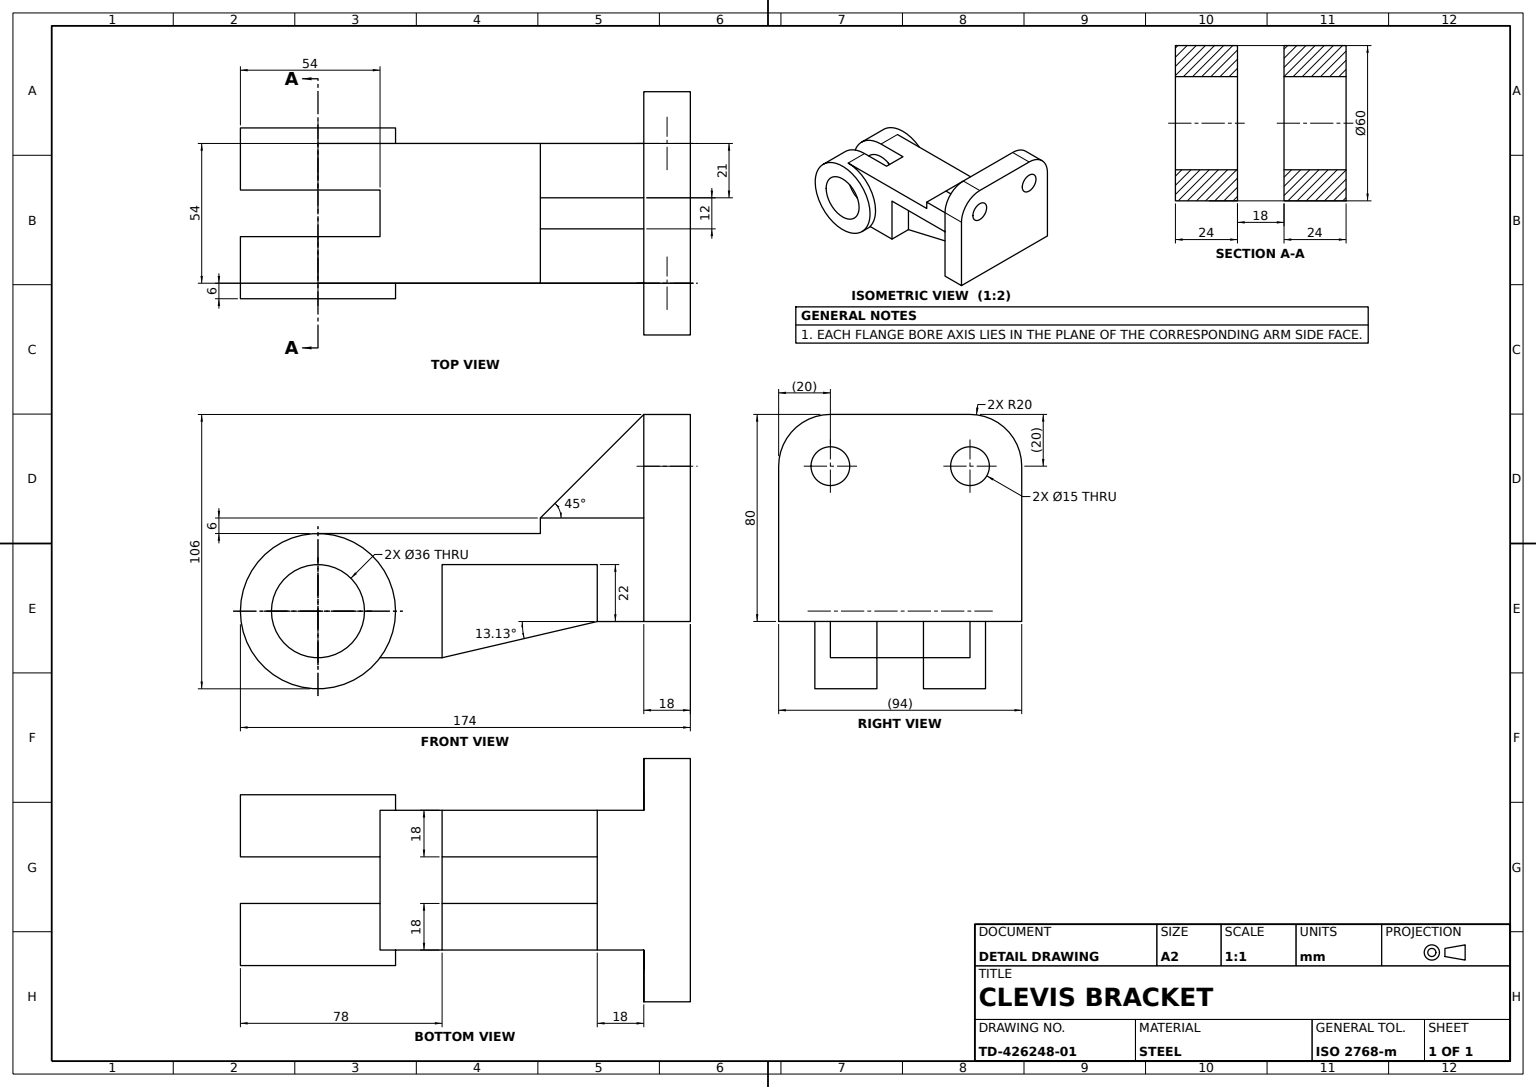
SolidWorks part; units mm, degrees
material "Plain Carbon Steel"
ref_plane "Front Plane" through (0, 0, 0) normal (0, 0, 1) x (1, 0, 0)
ref_plane "Top Plane" through (0, 0, 0) normal (0, 1, 0) x (1, 0, 0)
ref_plane "Right Plane" through (0, 0, 0) normal (1, 0, 0) x (0, 0, -1)
sketch "Clevis Lug A Sketch" plane through (0, 0, 0) normal (1, 0, 0) x (0, 0, -1)
  circle A0 centre (0, 0) radius 30
  circle A1 centre (0, 0) radius 18
  dimension "D1" = 36
  dimension "D2" = 60
extrude "Clevis Lug A Ø60xØ36" add sketch "Clevis Lug A Sketch" along normal blind 24
ref_plane "Plane1" through (-18, 0, 0) normal (1, 0, 0) x (0, 0, -1)
sketch "Clevis Lug B Sketch" plane through (-18, 0, 0) normal (1, 0, 0) x (0, 0, -1)
  circle A0 centre (0, 0) radius 18
  circle A1 centre (0, 0) radius 30
  dimension "D1" = 60
  dimension "D2" = 36
extrude "Clevis Lug B Ø60xØ36" add sketch "Clevis Lug B Sketch" against normal blind 24 separate body
ref_plane "Plane2" through (18, 0, 0) normal (1, 0, 0) x (0, 0, -1)
sketch "Arm Web Sketch" plane through (18, 0, 0) normal (1, 0, 0) x (0, 0, -1)
  line L0 (0, 30) -> (48, 30)
  line L1 (48, 30) -> (126, 30)
  line L2 (126, 30) -> (126, -4)
  line L3 (126, -4) -> (108, -4)
  line L4 (108, -4) -> (108, 18)
  line L5 (108, 18) -> (48, 18)
  line L6 (48, 18) -> (48, -4)
  line L7 (48, -4) -> (17.5499, -4)
  line L8 (0, 30) -> (0, 18)
  circle A0 centre (0, 0) radius 30 construction
  arc A1 (17.5499, -4) -> (0, 18) centre (0, 0) ccw
  dimension "D1" = 36
  dimension "D2" = 78
  dimension "D3" = 48
  dimension "D4" = 34
  dimension "D5" = 18
  dimension "D6" = 22
  dimension "D7" = 22
  dimension "D8" = 30.4501
extrude "Arm Web" add sketch "Arm Web Sketch" against normal blind 18
sketch "Lug Bridge Sketch" plane through (-18, 0, 0) normal (1, 0, 0) x (0, 0, -1)
  line L0 (0, 30) -> (126, 30)
  line L1 (126, 30) -> (126, -4)
  line L2 (126, -4) -> (108, -4)
  line L3 (108, -4) -> (108, 18)
  line L4 (108, 18) -> (48, 18)
  line L5 (48, 18) -> (48, -4)
  line L6 (48, -4) -> (17.5499, -4)
  line L7 (0, 30) -> (0, 18)
  circle A0 centre (0, 0) radius 30 construction
  arc A1 (17.5499, -4) -> (0, 18) centre (0, 0) ccw
  dimension "D1" = 18
extrude "Lug Bridge" add sketch "Lug Bridge Sketch" against normal blind 18
sketch "Arm Top Plate Sketch" plane through (0, 30, 0) normal (0, 1, 0) x (1, 0, 0)
  line L0 (18, 126) -> (18, 0) construction
  line L1 (-36, 126) -> (18, 126)
  line L2 (-36, 126) -> (-36, 86)
  line L3 (-36, 86) -> (18, 86)
  line L4 (18, 126) -> (18, 86)
  dimension "D1" = 40
extrude "Arm Top Plate 6mm" add sketch "Arm Top Plate Sketch" along normal blind 6
sketch "Arm Spine Sketch" plane through (18, 0, 0) normal (1, 0, 0) x (0, 0, -1)
  line L0 (0, 0) -> (4, 0)
  line L1 (24, -4) -> (48, -4)
  line L2 (48, -4) -> (48, 18)
  line L3 (24, -4) -> (24, 30)
  line L4 (86, 30) -> (0, 30) construction
  line L5 (24, 30) -> (126, 30)
  line L6 (126, 30) -> (126, 18)
  line L7 (126, -4) -> (126, 36) construction
  line L8 (126, 18) -> (48, 18)
  circle A0 centre (0, 0) radius 4
  arc M2 (0, 30) -> (29.7321, -4) centre (0, 0) cw
  line M3 (29.7321, -4) -> (48, -4)
  line M4 (48, -4) -> (48, 18)
  line M5 (48, 18) -> (108, 18)
  line M8 (126, -4) -> (126, 36)
  line M11 (86, 30) -> (0, 30)
  dimension "D1" = 24
extrude "Arm Spine 54mm" add sketch "Arm Spine Sketch" against normal blind 54 contours L8 L5 L3 M8 M11 M2 M3 M4 M5 | L3 L1 M2 | A0
sketch "Arm Body Sketch" plane through (0, 0, -126) normal (0, 0, -1) x (-1, 0, 0)
  line L1 (0, 18) -> (18, 18)
  line L2 (0, 18) -> (0, -4)
  line L3 (0, -4) -> (18, -4)
  line L4 (18, 18) -> (18, -4)
extrude "Arm Body 80mm" add sketch "Arm Body Sketch" against normal blind 80
sketch "Arm Side Web Sketch" plane through (18, 0, 0) normal (1, 0, 0) x (0, 0, -1)
  line L1 (48, -4) -> (48, -24)
  line L2 (48, -24) -> (24, -24)
  line L3 (24, -24) -> (24, 6)
  line L4 (48, 6) -> (48, -4)
  line L5 (48, -4) -> (48, 18) construction
  line L6 (24, 6) -> (48, 6)
  dimension "D1" = 20
  dimension "D2" = 24
  dimension "D3" = 10
extrude "Arm Side Web 54mm" add sketch "Arm Side Web Sketch" against normal blind 54
ref_plane "Plane3" through (-9, 0, 0) normal (1, 0, 0) x (0, 0, -1)
sketch "Arm Slot Sketch" plane through (-9, 0, 0) normal (1, 0, 0) x (0, 0, -1)
  line L0 (24, -24) -> (24, -18)
  line L1 (24, -18) -> (24, -24) construction
  line L2 (24, -18) -> (48, -18)
  line L3 (48, -24) -> (48, 18) construction
  line L4 (48, -18) -> (48, -24)
  line L5 (24, -24) -> (48, -24) construction
  line L6 (48, -24) -> (24, -24)
  circle A0 centre (0, 0) radius 30 construction
extrude "Arm Slot Cut" cut sketch "Arm Slot Sketch" against normal mid plane 54
sketch "Arm Rib Sketch" plane through (-9, 0, 0) normal (1, 0, 0) x (0, 0, -1)
  line L0 (48, -18) -> (108, -4)
rib "Arm Rib 18mm" sketch "Arm Rib Sketch" sketch "Arm Rib Sketch" thickness 18 extrusion direction parallel to sketch draft on no parameters "D1"=18
sketch "Mounting Flange Sketch" plane through (0, 0, -126) normal (0, 0, -1) x (-1, 0, 0)
  line L0 (-18, 36) -> (36, 36) construction
  line L1 (36, -4) -> (-18, -4) construction
  line L2 (-18, 76) -> (36, 76)
  line L3 (-38, 56) -> (-38, -4)
  line L4 (-38, -4) -> (56, -4)
  line L5 (56, -4) -> (56, 56)
  arc A0 (-18, 76) -> (-38, 56) centre (-18, 56) ccw
  circle A1 centre (-18, 56) radius 7.5
  circle A2 centre (36, 56) radius 7.5
  arc A3 (56, 56) -> (36, 76) centre (36, 56) ccw
  point P8 (9, 36)
  dimension "D1" = 40
  dimension "D2" = 15
  dimension "D3" = 15
  dimension "D4" = 40
  dimension "D5" = 27
  dimension "D6" = 27
  dimension "D7" = 60
  dimension "D8" = 60
  dimension "D9" = 60
  dimension "D10" = 54
extrude "Mounting Flange" add sketch "Mounting Flange Sketch" along normal blind 18
ref_plane "Plane4" through (-9, 0, 0) normal (1, 0, 0) x (0, 0, -1)
sketch "Flange Gusset Sketch" plane through (-9, 0, 0) normal (1, 0, 0) x (0, 0, -1)
  line L0 (86, 36) -> (126, 76)
rib "Flange Gusset 12mm" sketch "Flange Gusset Sketch" sketch "Flange Gusset Sketch" thickness 12 extrusion direction parallel to sketch draft on no parameters "D1"=12
